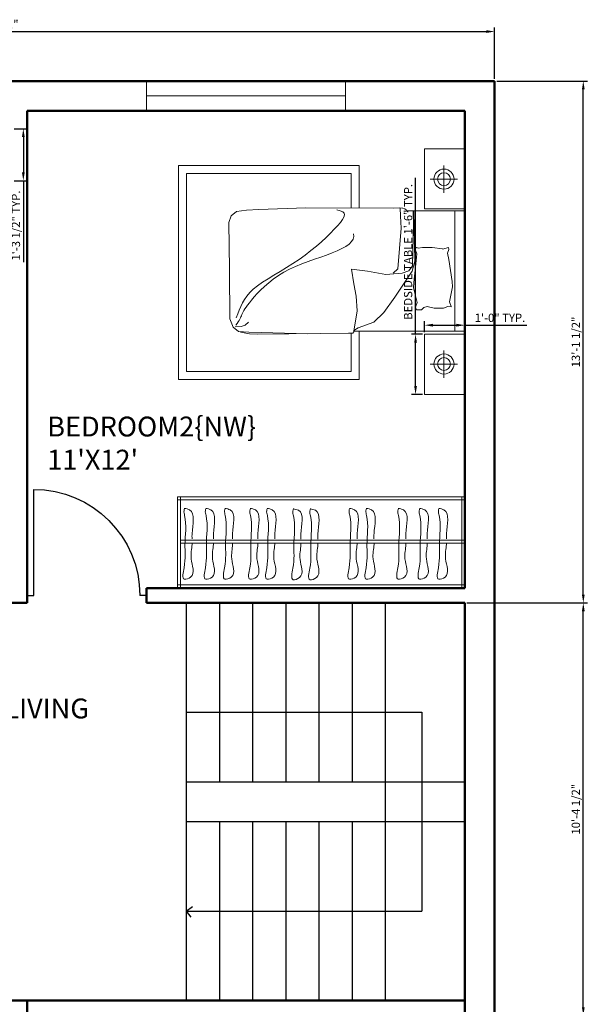
# Model space of a CAD drawing. Units: inches. Extents: x 20697 to 21575, y 6189 to 6822.
# Tile 7 of 7: x 21403 to 21575, y 6511 to 6808. Entities that reach past the tile are written whole.
import ezdxf

# ---------------------------------------------------------------- set-up
doc = ezdxf.new("R2010")
doc.units = ezdxf.units.IN
for name, color, linetype, lineweight in [('A-ANNO-DIMS', 2, 'Continuous', 18), ('A-AREA-IDEN', 7, 'Continuous', 18), ('A-DOOR', 4, 'Continuous', 25), ('A-FLOR-STRS', 3, 'Continuous', 25), ('A-FURN', 8, 'Continuous', 18), ('A-GLAZ', 4, 'Continuous', 18), ('A-WALL', 7, 'Continuous', 50)]:
    doc.layers.add(name, color=color, linetype=linetype, lineweight=lineweight)
doc.styles.get("Standard").update_dxf_attribs({"font": 'arial.ttf'})
doc.dimstyles.new('ISO-25', dxfattribs={"dimtxt": 2.5, "dimasz": 2.5, "dimexe": 1.25, "dimexo": 0.625, "dimtad": 1, "dimdec": 0, "dimlunit": 3, "dimtxsty": 'Standard', "dimcen": 2.5, "dimadec": 0, "dimazin": 0, "dimtfac": 1, "dimtdec": 0, "dimtmove": 0, "dimatfit": 3, "dimfxl": 1, "dimarcsym": 0})

# ---------------------------------------------------------------- blocks, each defined once
blk = doc.blocks.new('*D1')
at = {"layer": 'A-ANNO-DIMS', "color": 0, "lineweight": -2, "transparency": 16777216}
for p, q in [((21248.16, 6790.38), (21248.16, 6805.94)), ((21250.66, 6804.69), (21544.16, 6804.69)), ((21546.66, 6790.38), (21546.66, 6805.94))]:
    blk.add_line(p, q, dxfattribs=at)
at = {"layer": 'A-ANNO-DIMS', "color": 0, "transparency": 16777216}
for points in [[(21250.66, 6805.11), (21250.66, 6804.27), (21248.16, 6804.69)], [(21544.16, 6805.11), (21544.16, 6804.27), (21546.66, 6804.69)]]:
    blk.add_solid(points, dxfattribs=at)
at = {"layer": 'Defpoints', "color": 0, "transparency": 16777216}
for p in [(21546.66, 6804.69), (21248.16, 6789.76), (21546.66, 6789.76)]:
    blk.add_point(p, dxfattribs=at)
at = {"layer": 'A-ANNO-DIMS', "color": 0, "transparency": 16777216, "insert": (21397.41, 6806.57), "char_height": 2.5, "attachment_point": 5}
blk.add_mtext('24\'-11"', dxfattribs=at)
blk = doc.blocks.new('DOOR-SWING-36')
for p, q in [((34, 0), (34, 32)), ((0, 0), (2, 0)), ((36, 0), (34, 0))]:
    blk.add_line(p, q)
blk.add_arc((34, 0), 32, 90, 180)
blk = doc.blocks.new('WIN-60X9')
for p, q in [((0, 9), (60, 9)), ((0, 0), (0, 9)), ((60, 9), (60, 0)), ((0, 4.5), (60, 4.5)), ((60, 0), (0, 0))]:
    blk.add_line(p, q)
blk = doc.blocks.new('WARDROBE-HANGING')
for p, q in [((86.7, 27.55), (0, 27.55)), ((0, 27.55), (0, 0)), ((0.92, 27.55), (0.92, 0)), ((85.78, 27.55), (85.78, 0)), ((86.7, 27.55), (86.7, 0)), ((86.7, 26.63), (0, 26.63)), ((86.7, 14.43), (0.92, 14.43)), ((86.7, 13.51), (0.92, 13.51)), ((0, 0.92), (86.7, 0.92)), ((0, 0), (86.7, 0))]:
    blk.add_line(p, q)
for points, knots in [([(4.45, 13.46), (4.45, 13.37), (4.4, 11.87), (3.52, 8.61), (5.91, 3.75), (1.04, 1.92), (2.71, 8.17), (1.92, 13.34), (2.96, 19.5), (1.88, 23.12), (2.13, 23.84), (2.21, 24.08)], [256.949798, 256.949798, 256.949798, 256.949798, 263.372126, 359.428036, 478.655159, 522.640662, 597.66786, 752.004169, 941.88133, 973.527729, 990.309099, 990.309099, 990.309099, 990.309099]), ([(2.11, 24.03), (2.69, 23.93), (5.79, 23.36), (4.37, 18.34), (4.42, 15.35), (4.44, 14.84)], [0, 0, 0, 0, 35.911014, 192.421107, 225.897258, 225.897258, 225.897258, 225.897258]), ([(10.89, 13.46), (10.89, 13.37), (10.83, 11.87), (9.95, 8.61), (12.35, 3.75), (7.48, 1.92), (9.15, 8.17), (8.36, 13.34), (9.4, 19.5), (8.32, 23.12), (8.56, 23.84), (8.65, 24.08)], [256.949798, 256.949798, 256.949798, 256.949798, 263.372126, 359.428036, 478.655159, 522.640662, 597.66786, 752.004169, 941.88133, 973.527729, 990.309099, 990.309099, 990.309099, 990.309099]), ([(8.55, 24.03), (9.13, 23.93), (12.23, 23.36), (10.8, 18.34), (10.86, 15.35), (10.87, 14.84)], [0, 0, 0, 0, 35.911014, 192.421107, 225.897258, 225.897258, 225.897258, 225.897258]), ([(16.68, 13.46), (16.68, 13.37), (16.63, 11.87), (15.75, 8.61), (18.14, 3.75), (13.27, 1.92), (14.94, 8.17), (14.15, 13.34), (15.19, 19.5), (14.11, 23.12), (14.36, 23.84), (14.44, 24.08)], [256.949798, 256.949798, 256.949798, 256.949798, 263.372126, 359.428036, 478.655159, 522.640662, 597.66786, 752.004169, 941.88133, 973.527729, 990.309099, 990.309099, 990.309099, 990.309099]), ([(14.34, 24.03), (14.92, 23.93), (18.02, 23.36), (16.6, 18.34), (16.65, 15.35), (16.67, 14.84)], [0, 0, 0, 0, 35.911014, 192.421107, 225.897258, 225.897258, 225.897258, 225.897258]), ([(24.29, 13.46), (24.29, 13.37), (24.23, 11.87), (23.36, 8.61), (25.75, 3.75), (20.88, 1.92), (22.55, 8.17), (21.76, 13.34), (22.8, 19.5), (21.72, 23.12), (21.96, 23.84), (22.05, 24.08)], [256.949798, 256.949798, 256.949798, 256.949798, 263.372126, 359.428036, 478.655159, 522.640662, 597.66786, 752.004169, 941.88133, 973.527729, 990.309099, 990.309099, 990.309099, 990.309099]), ([(21.95, 24.03), (22.53, 23.93), (25.63, 23.36), (24.2, 18.34), (24.26, 15.35), (24.27, 14.84)], [0, 0, 0, 0, 35.911014, 192.421107, 225.897258, 225.897258, 225.897258, 225.897258]), ([(29.4, 13.46), (29.39, 13.37), (29.34, 11.87), (28.46, 8.61), (30.85, 3.75), (25.99, 1.92), (27.66, 8.17), (26.86, 13.34), (27.9, 19.5), (26.82, 23.12), (27.07, 23.84), (27.15, 24.08)], [256.949798, 256.949798, 256.949798, 256.949798, 263.372126, 359.428036, 478.655159, 522.640662, 597.66786, 752.004169, 941.88133, 973.527729, 990.309099, 990.309099, 990.309099, 990.309099]), ([(27.05, 24.03), (27.63, 23.93), (30.74, 23.36), (29.31, 18.34), (29.37, 15.35), (29.38, 14.84)], [0, 0, 0, 0, 35.911014, 192.421107, 225.897258, 225.897258, 225.897258, 225.897258]), ([(37.29, 13.32), (37.28, 13.23), (37.23, 11.74), (36.35, 8.47), (38.74, 3.62), (33.88, 1.78), (35.55, 8.04), (34.75, 13.2), (35.79, 19.36), (34.71, 22.98), (34.96, 23.7), (35.04, 23.95)], [256.949798, 256.949798, 256.949798, 256.949798, 263.372126, 359.428036, 478.655159, 522.640662, 597.66786, 752.004169, 941.88133, 973.527729, 990.309099, 990.309099, 990.309099, 990.309099]), ([(34.94, 23.9), (35.52, 23.79), (38.63, 23.22), (37.2, 18.2), (37.26, 15.21), (37.27, 14.7)], [0, 0, 0, 0, 35.911014, 192.421107, 225.897258, 225.897258, 225.897258, 225.897258]), ([(42.39, 13.32), (42.39, 13.23), (42.33, 11.74), (41.46, 8.47), (43.85, 3.62), (38.98, 1.78), (40.65, 8.04), (39.86, 13.2), (40.9, 19.36), (39.82, 22.98), (40.06, 23.7), (40.15, 23.95)], [256.949798, 256.949798, 256.949798, 256.949798, 263.372126, 359.428036, 478.655159, 522.640662, 597.66786, 752.004169, 941.88133, 973.527729, 990.309099, 990.309099, 990.309099, 990.309099]), ([(40.05, 23.9), (40.63, 23.79), (43.73, 23.22), (42.3, 18.2), (42.36, 15.21), (42.38, 14.7)], [0, 0, 0, 0, 35.911014, 192.421107, 225.897258, 225.897258, 225.897258, 225.897258]), ([(54.23, 13.46), (54.23, 13.37), (54.17, 11.87), (53.3, 8.61), (55.69, 3.75), (50.82, 1.92), (52.49, 8.17), (51.7, 13.34), (52.74, 19.5), (51.66, 23.12), (51.9, 23.84), (51.99, 24.08)], [256.949798, 256.949798, 256.949798, 256.949798, 263.372126, 359.428036, 478.655159, 522.640662, 597.66786, 752.004169, 941.88133, 973.527729, 990.309099, 990.309099, 990.309099, 990.309099]), ([(51.89, 24.03), (52.47, 23.93), (55.57, 23.36), (54.14, 18.34), (54.2, 15.35), (54.22, 14.84)], [0, 0, 0, 0, 35.911014, 192.421107, 225.897258, 225.897258, 225.897258, 225.897258]), ([(59.34, 13.46), (59.33, 13.37), (59.28, 11.87), (58.4, 8.61), (60.79, 3.75), (55.93, 1.92), (57.6, 8.17), (56.8, 13.34), (57.84, 19.5), (56.76, 23.12), (57.01, 23.84), (57.09, 24.08)], [256.949798, 256.949798, 256.949798, 256.949798, 263.372126, 359.428036, 478.655159, 522.640662, 597.66786, 752.004169, 941.88133, 973.527729, 990.309099, 990.309099, 990.309099, 990.309099]), ([(56.99, 24.03), (57.57, 23.93), (60.68, 23.36), (59.25, 18.34), (59.31, 15.35), (59.32, 14.84)], [0, 0, 0, 0, 35.911014, 192.421107, 225.897258, 225.897258, 225.897258, 225.897258]), ([(68.95, 13.46), (68.95, 13.37), (68.89, 11.87), (68.01, 8.61), (70.41, 3.75), (65.54, 1.92), (67.21, 8.17), (66.42, 13.34), (67.46, 19.5), (66.38, 23.12), (66.62, 23.84), (66.71, 24.08)], [256.949798, 256.949798, 256.949798, 256.949798, 263.372126, 359.428036, 478.655159, 522.640662, 597.66786, 752.004169, 941.88133, 973.527729, 990.309099, 990.309099, 990.309099, 990.309099]), ([(66.61, 24.03), (67.19, 23.93), (70.29, 23.36), (68.86, 18.34), (68.92, 15.35), (68.93, 14.84)], [0, 0, 0, 0, 35.911014, 192.421107, 225.897258, 225.897258, 225.897258, 225.897258]), ([(75.39, 13.46), (75.38, 13.37), (75.33, 11.87), (74.45, 8.61), (76.84, 3.75), (71.98, 1.92), (73.65, 8.17), (72.85, 13.34), (73.89, 19.5), (72.81, 23.12), (73.06, 23.84), (73.14, 24.08)], [256.949798, 256.949798, 256.949798, 256.949798, 263.372126, 359.428036, 478.655159, 522.640662, 597.66786, 752.004169, 941.88133, 973.527729, 990.309099, 990.309099, 990.309099, 990.309099]), ([(73.04, 24.03), (73.62, 23.93), (76.73, 23.36), (75.3, 18.34), (75.36, 15.35), (75.37, 14.84)], [0, 0, 0, 0, 35.911014, 192.421107, 225.897258, 225.897258, 225.897258, 225.897258]), ([(81.18, 13.46), (81.18, 13.37), (81.12, 11.87), (80.24, 8.61), (82.64, 3.75), (77.77, 1.92), (79.44, 8.17), (78.65, 13.34), (79.69, 19.5), (78.61, 23.12), (78.85, 23.84), (78.94, 24.08)], [256.949798, 256.949798, 256.949798, 256.949798, 263.372126, 359.428036, 478.655159, 522.640662, 597.66786, 752.004169, 941.88133, 973.527729, 990.309099, 990.309099, 990.309099, 990.309099]), ([(78.84, 24.03), (79.42, 23.93), (82.52, 23.36), (81.09, 18.34), (81.15, 15.35), (81.16, 14.84)], [0, 0, 0, 0, 35.911014, 192.421107, 225.897258, 225.897258, 225.897258, 225.897258])]:
    blk.add_open_spline(points, degree=3, knots=knots)
blk = doc.blocks.new('NIGHTSTAND-WITH-LAMP-LARGE')
for p, q in [((5.85, 5.06), (5.85, 13.3)), ((9.97, 9.18), (1.73, 9.18))]:
    blk.add_line(p, q)
blk.add_lwpolyline([(0, 0), (0, 18.17), (12.12, 18.17), (12.12, 0)], close=True)
for radius in [3.03, 1.94]:
    blk.add_circle((5.85, 9.18), radius)
blk = doc.blocks.new('*D35')
at = {"layer": 'A-ANNO-DIMS', "color": 0, "lineweight": -2, "transparency": 16777216}
for p, q in [((21401.79, 6775.38), (21405.76, 6775.38)), ((21404.51, 6772.88), (21404.51, 6762.18)), ((21401.79, 6759.68), (21405.76, 6759.68)), ((21404.51, 6759.68), (21404.51, 6735.1))]:
    blk.add_line(p, q, dxfattribs=at)
at = {"layer": 'A-ANNO-DIMS', "color": 0, "transparency": 16777216}
for points in [[(21404.09, 6772.88), (21404.93, 6772.88), (21404.51, 6775.38)], [(21404.09, 6762.18), (21404.93, 6762.18), (21404.51, 6759.68)]]:
    blk.add_solid(points, dxfattribs=at)
at = {"layer": 'Defpoints', "color": 0, "transparency": 16777216}
for p in [(21401.16, 6775.38), (21401.16, 6759.68), (21404.51, 6759.68)]:
    blk.add_point(p, dxfattribs=at)
at = {"layer": 'A-ANNO-DIMS', "color": 0, "transparency": 16777216, "insert": (21402.59, 6746.14), "char_height": 2.5, "attachment_point": 5, "rotation": 90}
blk.add_mtext('1\'-3 1/2" TYP.', dxfattribs=at)
blk = doc.blocks.new('*D42')
at = {"layer": 'A-ANNO-DIMS', "color": 0, "lineweight": -2, "transparency": 16777216}
for p, q in [((21522.82, 6713.35), (21522.82, 6760.57)), ((21524.92, 6713.35), (21521.57, 6713.35)), ((21522.82, 6697.68), (21522.82, 6710.85)), ((21524.92, 6695.18), (21521.57, 6695.18))]:
    blk.add_line(p, q, dxfattribs=at)
at = {"layer": 'A-ANNO-DIMS', "color": 0, "transparency": 16777216}
for points in [[(21522.4, 6710.85), (21523.23, 6710.85), (21522.82, 6713.35)], [(21522.4, 6697.68), (21523.23, 6697.68), (21522.82, 6695.18)]]:
    blk.add_solid(points, dxfattribs=at)
at = {"layer": 'Defpoints', "color": 0, "transparency": 16777216}
for p in [(21522.82, 6713.35), (21525.54, 6713.35), (21525.54, 6695.18)]:
    blk.add_point(p, dxfattribs=at)
at = {"layer": 'A-ANNO-DIMS', "color": 0, "transparency": 16777216, "insert": (21520.9, 6738.21), "char_height": 2.5, "attachment_point": 5, "rotation": 90}
blk.add_mtext('BEDSIDE TABLE 1\'-6" TYP.', dxfattribs=at)
blk = doc.blocks.new('*D43')
at = {"layer": 'A-ANNO-DIMS', "color": 0, "lineweight": -2, "transparency": 16777216}
for p, q in [((21525.54, 6713.98), (21525.54, 6717.33)), ((21528.04, 6716.08), (21535.16, 6716.08)), ((21537.66, 6713.98), (21537.66, 6717.33)), ((21537.66, 6716.08), (21556.41, 6716.08))]:
    blk.add_line(p, q, dxfattribs=at)
at = {"layer": 'A-ANNO-DIMS', "color": 0, "transparency": 16777216}
for points in [[(21528.04, 6716.5), (21528.04, 6715.66), (21525.54, 6716.08)], [(21535.16, 6716.5), (21535.16, 6715.66), (21537.66, 6716.08)]]:
    blk.add_solid(points, dxfattribs=at)
at = {"layer": 'Defpoints', "color": 0, "transparency": 16777216}
for p in [(21537.66, 6716.08), (21525.54, 6713.35), (21537.66, 6713.35)]:
    blk.add_point(p, dxfattribs=at)
at = {"layer": 'A-ANNO-DIMS', "color": 0, "transparency": 16777216, "insert": (21548.28, 6717.98), "char_height": 2.5, "attachment_point": 5}
blk.add_mtext('1\'-0" TYP.', dxfattribs=at)
blk = doc.blocks.new('*D66')
at = {"layer": 'A-ANNO-DIMS', "color": 0, "lineweight": -2, "transparency": 16777216}
for p, q in [((21538.29, 6632.26), (21574.66, 6632.26)), ((21573.41, 6510.26), (21573.41, 6629.76)), ((21538.29, 6507.76), (21574.66, 6507.76))]:
    blk.add_line(p, q, dxfattribs=at)
at = {"layer": 'A-ANNO-DIMS', "color": 0, "transparency": 16777216}
for points in [[(21573, 6629.76), (21573.83, 6629.76), (21573.41, 6632.26)], [(21573, 6510.26), (21573.83, 6510.26), (21573.41, 6507.76)]]:
    blk.add_solid(points, dxfattribs=at)
at = {"layer": 'Defpoints', "color": 0, "transparency": 16777216}
for p in [(21537.66, 6632.26), (21573.41, 6632.26), (21537.66, 6507.76)]:
    blk.add_point(p, dxfattribs=at)
at = {"layer": 'A-ANNO-DIMS', "color": 0, "transparency": 16777216, "insert": (21571.49, 6570.01), "char_height": 2.5, "attachment_point": 5, "rotation": 90}
blk.add_mtext('10\'-4 1/2"', dxfattribs=at)
blk = doc.blocks.new('*D67')
at = {"layer": 'A-ANNO-DIMS', "color": 0, "lineweight": -2, "transparency": 16777216}
for p, q in [((21547.29, 6789.76), (21574.66, 6789.76)), ((21573.41, 6634.76), (21573.41, 6787.26)), ((21538.29, 6632.26), (21574.66, 6632.26))]:
    blk.add_line(p, q, dxfattribs=at)
at = {"layer": 'A-ANNO-DIMS', "color": 0, "transparency": 16777216}
for points in [[(21573, 6787.26), (21573.83, 6787.26), (21573.41, 6789.76)], [(21573, 6634.76), (21573.83, 6634.76), (21573.41, 6632.26)]]:
    blk.add_solid(points, dxfattribs=at)
at = {"layer": 'Defpoints', "color": 0, "transparency": 16777216}
for p in [(21546.66, 6789.76), (21573.41, 6789.76), (21537.66, 6632.26)]:
    blk.add_point(p, dxfattribs=at)
at = {"layer": 'A-ANNO-DIMS', "color": 0, "transparency": 16777216, "insert": (21571.49, 6711.01), "char_height": 2.5, "attachment_point": 5, "rotation": 90}
blk.add_mtext('13\'-1 1/2"', dxfattribs=at)

msp = doc.modelspace()

# ---------------------------------------------------------------- linework, layer by layer
at = {"layer": 'A-FLOR-STRS'}
for p, q in [((21453.66, 6632.26), (21453.66, 6566.26)), ((21463.66, 6632.26), (21463.66, 6578.26)), ((21473.66, 6632.26), (21473.66, 6578.26)), ((21483.66, 6632.26), (21483.66, 6578.26)), ((21493.66, 6632.26), (21493.66, 6578.26)), ((21503.66, 6632.26), (21503.66, 6578.26)), ((21513.66, 6632.26), (21513.66, 6512.26)), ((21453.66, 6599.26), (21524.66, 6599.26)), ((21524.66, 6599.26), (21524.66, 6539.26)), ((21453.66, 6578.26), (21513.66, 6578.26)), ((21513.66, 6578.26), (21537.66, 6578.26)), ((21453.66, 6566.26), (21513.66, 6566.26)), ((21453.66, 6566.26), (21453.66, 6512.26)), ((21463.66, 6566.26), (21463.66, 6512.26)), ((21473.66, 6566.26), (21473.66, 6512.26)), ((21483.66, 6566.26), (21483.66, 6512.26)), ((21493.66, 6566.26), (21493.66, 6512.26)), ((21503.66, 6566.26), (21503.66, 6512.26)), ((21513.66, 6566.26), (21537.66, 6566.26)), ((21453.66, 6539.26), (21455.49, 6540.61)), ((21453.66, 6539.26), (21524.66, 6539.26)), ((21453.66, 6539.26), (21455.04, 6537.39))]:
    msp.add_line(p, q, dxfattribs=at)
at = {"layer": 'A-FURN'}
for p, q in [((21451.28, 6699.66), (21451.28, 6764.23)), ((21451.28, 6764.23), (21505.8, 6764.23)), ((21505.8, 6764.23), (21505.8, 6751.46)), ((21453.71, 6702.08), (21453.71, 6761.81)), ((21453.71, 6761.81), (21503.38, 6761.81)), ((21503.38, 6761.81), (21503.38, 6751.47)), ((21489.71, 6751.53), (21475.55, 6750.96)), ((21516.1, 6751.42), (21489.71, 6751.53)), ((21518.08, 6751.45), (21516.1, 6751.42)), ((21518.93, 6751.37), (21518.08, 6751.45)), ((21467.18, 6749.1), (21466.5, 6747.08)), ((21468.8, 6750.43), (21467.18, 6749.1)), ((21471.85, 6750.77), (21468.8, 6750.43)), ((21475.55, 6750.96), (21471.85, 6750.77)), ((21520.13, 6750.6), (21537.66, 6750.6)), ((21534.63, 6714.26), (21534.63, 6750.54)), ((21466.5, 6747.08), (21466.66, 6732.89)), ((21530.99, 6739.07), (21532.75, 6739.54)), ((21466.66, 6732.89), (21466.66, 6726.39)), ((21522.15, 6727.35), (21522.26, 6729.01)), ((21523.28, 6722.93), (21522.15, 6727.35)), ((21533.06, 6723.15), (21533.99, 6727.61)), ((21533.99, 6727.61), (21533.81, 6729.26)), ((21466.66, 6726.39), (21466.83, 6724.08)), ((21466.83, 6724.08), (21466.83, 6718.01)), ((21522.84, 6721.53), (21523.28, 6722.93)), ((21523.11, 6720.67), (21522.84, 6721.53)), ((21525.36, 6721.37), (21524.57, 6720.76)), ((21526.35, 6721.71), (21525.36, 6721.37)), ((21528.41, 6721.22), (21526.35, 6721.71)), ((21532.51, 6721.74), (21531.2, 6721.19)), ((21533.53, 6721.64), (21532.51, 6721.74)), ((21533.53, 6721.64), (21532.51, 6721.74)), ((21533.57, 6721.77), (21533.06, 6723.15)), ((21533.53, 6721.64), (21533.57, 6721.77)), ((21524.57, 6720.76), (21523.11, 6720.67)), ((21531.2, 6721.19), (21528.41, 6721.22)), ((21467.78, 6715.45), (21466.83, 6718.01)), ((21469.43, 6714.17), (21467.78, 6715.45)), ((21468.4, 6715.57), (21470.2, 6715.66)), ((21470.2, 6715.66), (21471.45, 6716.06)), ((21471.45, 6716.06), (21472.38, 6716.95)), ((21472.49, 6713.93), (21469.43, 6714.17)), ((21469.99, 6714.02), (21472.69, 6713.5)), ((21476.2, 6713.85), (21472.49, 6713.93)), ((21472.69, 6713.5), (21475.29, 6713.35)), ((21475.29, 6713.35), (21494.04, 6713.54)), ((21490.37, 6713.48), (21476.2, 6713.85)), ((21494.04, 6713.54), (21502.61, 6713.63)), ((21503.38, 6713.68), (21503.38, 6702.08)), ((21504.2, 6714.35), (21504.25, 6714.24)), ((21504.3, 6714.26), (21537.66, 6714.26)), ((21505.8, 6714.26), (21505.8, 6699.66)), ((21503.38, 6702.08), (21453.71, 6702.08)), ((21505.8, 6699.66), (21451.28, 6699.66))]:
    msp.add_line(p, q, dxfattribs=at)
for points in [[(21516.06, 6731.73), (21517.46, 6733.1), (21518.5, 6745.4), (21518.29, 6748.99), (21518.17, 6751.45)], [(21518.98, 6751.34), (21519.55, 6751.17), (21519.98, 6750.91), (21520.13, 6750.6), (21520.44, 6750.25), (21520.46, 6750.19)], [(21468.67, 6718.32), (21469.17, 6719.48), (21469.64, 6720.61), (21470.11, 6721.7), (21470.61, 6722.78), (21471.2, 6723.83), (21471.91, 6724.88), (21472.78, 6725.91), (21473.85, 6726.95), (21475.15, 6727.99), (21476.65, 6729.04), (21478.31, 6730.11), (21480.1, 6731.2), (21481.97, 6732.33), (21483.89, 6733.49), (21485.81, 6734.69), (21487.7, 6735.94), (21489.53, 6737.24), (21491.27, 6738.58), (21492.91, 6739.93), (21494.45, 6741.27), (21495.87, 6742.57), (21497.16, 6743.83), (21498.31, 6745.02), (21499.31, 6746.11), (21500.13, 6747.09), (21500.77, 6747.95), (21501.19, 6748.7), (21501.36, 6749.34), (21501.25, 6749.88), (21500.85, 6750.31), (21500.12, 6750.63), (21499.03, 6750.85)], [(21504.17, 6714.26), (21505.24, 6720.37), (21504.9, 6724.88), (21504.16, 6728.57), (21503.54, 6732.94), (21508.32, 6732.35), (21513.87, 6731.37), (21518.77, 6731.8), (21520.75, 6732.44), (21521.89, 6734.04), (21522.24, 6746.96), (21522.13, 6750.6)], [(21522.25, 6750.6), (21522.55, 6735.42), (21521.78, 6732.39), (21518.56, 6727.55), (21516.55, 6724.51), (21513.2, 6719.94), (21510.23, 6717.02), (21505.46, 6715.31), (21504.21, 6714.46)], [(21534.63, 6714.26), (21534.63, 6750.6)], [(21537.66, 6750.6), (21537.66, 6714.26)], [(21468.6, 6716.11), (21468.98, 6716.62), (21469.3, 6717.08), (21469.56, 6717.5), (21469.78, 6717.88), (21469.97, 6718.25), (21470.13, 6718.6), (21470.29, 6718.95), (21470.44, 6719.3), (21470.61, 6719.67), (21470.8, 6720.06), (21471.04, 6720.49), (21471.33, 6720.98), (21471.7, 6721.52), (21472.14, 6722.15), (21472.69, 6722.86), (21473.35, 6723.67), (21474.13, 6724.59), (21475.04, 6725.6), (21476.07, 6726.67), (21477.23, 6727.77), (21478.51, 6728.89), (21479.91, 6730), (21481.43, 6731.06), (21483.06, 6732.06), (21484.81, 6732.97), (21486.65, 6733.81), (21488.54, 6734.58), (21490.45, 6735.3), (21492.35, 6735.97), (21494.2, 6736.62), (21495.99, 6737.26), (21497.66, 6737.89), (21499.2, 6738.53), (21500.58, 6739.19), (21501.78, 6739.87), (21502.76, 6740.57), (21503.51, 6741.29), (21504.01, 6742.05), (21504.22, 6742.84), (21504.12, 6743.67)], [(21522.26, 6729.01), (21522.95, 6735.64), (21523.19, 6737.57), (21522.77, 6738.69), (21522.89, 6739.61), (21523.63, 6739.36), (21524.88, 6739.51), (21527.8, 6739.56), (21530.99, 6739.14)], [(21533.81, 6729.26), (21532.82, 6735.86), (21532.5, 6737.77), (21532.86, 6738.91), (21532.75, 6739.54)], [(21502.69, 6713.63), (21503.87, 6713.71), (21504.22, 6714.06), (21504.3, 6714.26)]]:
    msp.add_lwpolyline(points, dxfattribs=at)
at = {"layer": 'A-WALL'}
for p, q in [((21248.16, 6789.76), (21546.66, 6789.76)), ((21546.66, 6789.76), (21546.66, 6330.76)), ((21405.66, 6780.76), (21405.66, 6632.26)), ((21405.66, 6780.76), (21537.66, 6780.76)), ((21537.66, 6780.76), (21537.66, 6636.76)), ((21441.66, 6634.51), (21441.66, 6636.76)), ((21441.66, 6636.76), (21537.66, 6636.76)), ((21401.16, 6632.26), (21405.66, 6632.26)), ((21441.66, 6634.51), (21441.66, 6632.26)), ((21441.66, 6632.26), (21537.66, 6632.26)), ((21537.66, 6632.26), (21537.66, 6392.26)), ((21401.16, 6512.26), (21537.66, 6512.26)), ((21405.66, 6512.26), (21405.66, 6392.26))]:
    msp.add_line(p, q, dxfattribs=at)

# ---------------------------------------------------------------- block references
at = {"layer": 'A-DOOR', "extrusion": (0, 0, -1), "zscale": -1}
msp.add_blockref('DOOR-SWING-36', (-21441.66, 6634.51), dxfattribs=at)
at = {"layer": 'A-FURN', "extrusion": (0, 0, -1), "zscale": -1, "rotation": 180}
msp.add_blockref('NIGHTSTAND-WITH-LAMP-LARGE', (-21525.54, 6769.33), dxfattribs=at)
at = {"layer": 'A-FURN'}
for name, p in [('NIGHTSTAND-WITH-LAMP-LARGE', (21525.54, 6695.18)), ('WARDROBE-HANGING', (21450.96, 6636.76))]:
    msp.add_blockref(name, p, dxfattribs=at)
at = {"layer": 'A-GLAZ'}
msp.add_blockref('WIN-60X9', (21441.66, 6780.76), dxfattribs=at)

# ---------------------------------------------------------------- texts
at = {"layer": 'A-AREA-IDEN', "char_height": 6, "attachment_point": 1}
for s, insert in [("BEDROOM2\\{NW\\}\\P11'X12'", (21411.71, 6688.49)), ("FAMILY LIVING\\P10'X12'", (21369.63, 6603.41))]:
    msp.add_mtext(s, dxfattribs=dict(at, insert=insert))

# ---------------------------------------------------------------- dimensions: what is measured, and where the dimension line sits
at = {"layer": 'A-ANNO-DIMS'}
dim = msp.add_linear_dim(base=(21546.66169726, 6804.69035485), p1=(21248.16169726, 6789.75667437), p2=(21546.66169726, 6789.75667437), dimstyle='ISO-25', override={"dimclrd": 0, "dimclre": 0, "dimclrt": 0}, dxfattribs=at)
dim.commit()
dim.dimension.update_dxf_attribs({"geometry": '*D1', "text_midpoint": (21397.41169726, 6806.57047082)})
for base, p1, p2, picture, middle in [((21573.41, 6789.76), (21537.66, 6632.26), (21546.66, 6789.76), '*D67', (21571.49, 6711.01)), ((21573.41, 6632.26), (21537.66, 6507.76), (21537.66, 6632.26), '*D66', (21571.49, 6570.01))]:
    dim = msp.add_linear_dim(base=base, p1=p1, p2=p2, angle=90, dimstyle='ISO-25', override={"dimdec": 1, "dimlfac": 1, "dimrnd": 0, "dimzin": 1, "dimdsep": 46, "dimlunit": 4, "dimfrac": 2}, dxfattribs=at)
    dim.commit()
    dim.dimension.update_dxf_attribs({"geometry": picture, "text_midpoint": middle})
for base, p1, p2, angle, text, picture, middle in [((21404.51, 6759.68), (21401.16, 6775.38), (21401.16, 6759.68), 270, '<> TYP.', '*D35', (21402.59, 6746.14)), ((21522.82, 6713.35), (21525.54, 6695.18), (21525.54, 6713.35), 90, 'BEDSIDE TABLE <> TYP.', '*D42', (21520.9, 6738.21))]:
    dim = msp.add_linear_dim(base=base, p1=p1, p2=p2, angle=angle, text=text, dimstyle='ISO-25', override={"dimdec": 1, "dimlfac": 1, "dimrnd": 0, "dimzin": 1, "dimdsep": 46, "dimlunit": 4, "dimfrac": 2}, dxfattribs=at)
    dim.commit()
    dim.dimension.update_dxf_attribs({"geometry": picture, "text_midpoint": middle})
dim = msp.add_linear_dim(base=(21537.66, 6716.08), p1=(21525.54, 6713.35), p2=(21537.66, 6713.35), text='<> TYP.', dimstyle='ISO-25', override={"dimdec": 1, "dimlfac": 1, "dimrnd": 0, "dimzin": 1, "dimdsep": 46, "dimlunit": 4, "dimfrac": 2}, dxfattribs=at)
dim.commit()
dim.dimension.update_dxf_attribs({"geometry": '*D43', "text_midpoint": (21548.28, 6717.98)})

doc.saveas('drawing.dxf')
